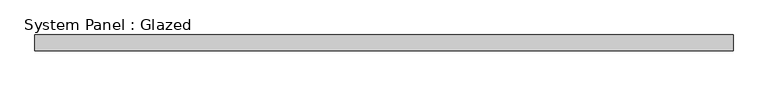
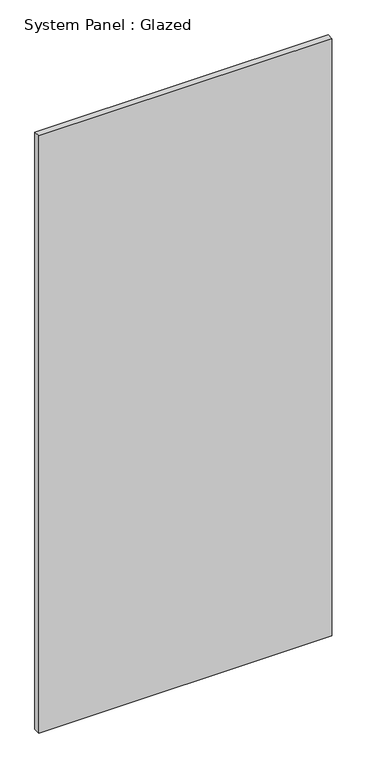
"""IFC4 building model written with IfcOpenShell, lengths in millimetres: plate geometry, System Panel : Glazed."""

from ifc_helpers import new_model, si_unit, origin, origin_with_axes, place, context, project, spatial, polyline, outline, extrude, source, transform, mapped, element, save


def system_panel_glazed_47378ea7(model_context):
    return source(origin(), model_context, "Body", "SweptSolid", [
        extrude(outline(polyline([(566.2083333, 19.05), (-566.2083333, 19.05), (-566.2083333, 44.45), (566.2083333, 44.45), (566.2083333, 19.05)])), origin_with_axes(), (0.0, 0.0, 1.0), 2438.4),
    ])


if __name__ == "__main__":
    model = new_model("IFC4")
    model_context = context("Model", 3, world=origin())
    ifc_project = project(units=[si_unit("LENGTHUNIT", "METRE", prefix="MILLI")], contexts=[model_context])
    site = spatial("IfcSite", under=ifc_project)
    building = spatial("IfcBuilding", under=site)
    placement = place(None, origin())
    system_panel_glazed_shape = system_panel_glazed_47378ea7(model_context)
    element("IfcPlate", 1, ObjectType="System Panel : Glazed", at=placement, inside=building, context=model_context, shape_type="MappedRepresentation", body=[
        mapped(system_panel_glazed_shape, transform((0.0, 0.0, 0.0), x_axis=(1.0, 0.0, 0.0), y_axis=(0.0, 1.0, 0.0), z_axis=(0.0, 0.0, 1.0))),
    ])
    save(model, "model.ifc")

# Revit data of these elements
# Type "System Panel : Glazed"
#   Construction Type Id = "GSP4R"
#   Analytic Construction = "1/8 in Pilkington single glazing"
#   Visual Light Transmittance = 0.9
#   Solar Heat Gain Coefficient = 0.86
#   Heat Transfer Coefficient (U) = 1.18115 BTU/(h·ft²·°F)
# Element 1 (IfcPlate, "System Panel : Glazed")
#   Materials on its faces: "Glass"
# Materials
#   "Glass": class "Glass", colour RGB 0 128 192, transparency 0.75, Description = "Soda Lime Glass", Cost = 0
